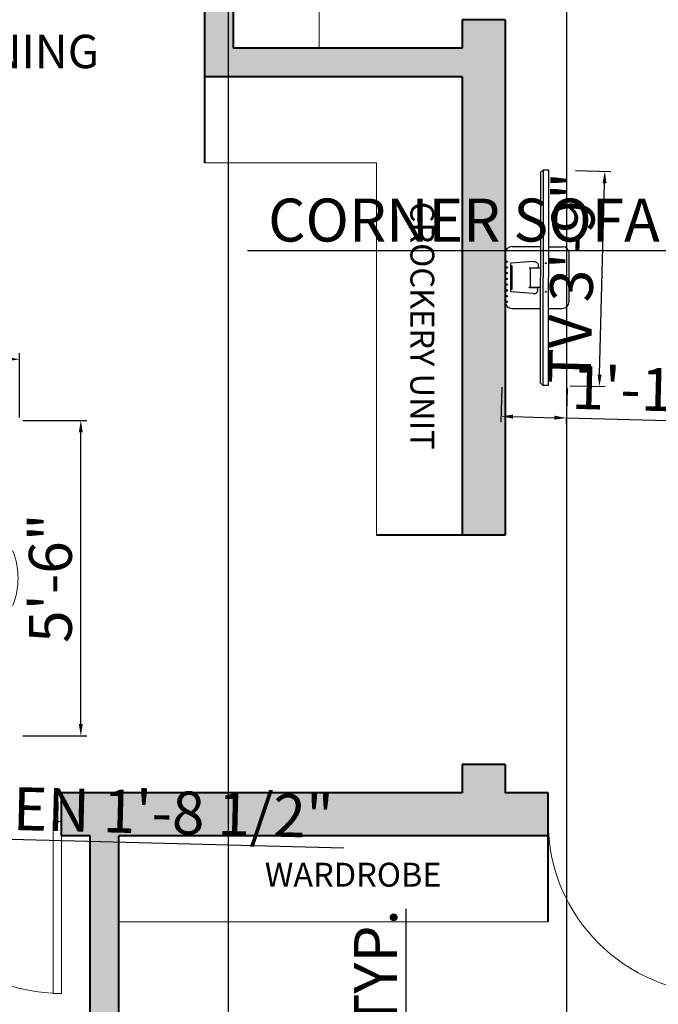
# Model space of a CAD drawing. Units: inches. Extents: x 2337 to 3570, y 1258 to 1938.
# Tile 4 of 30: x 2570 to 2704, y 1507 to 1713. Entities that reach past the tile are written whole.
import ezdxf

# ---------------------------------------------------------------- set-up
doc = ezdxf.new("R2010")
doc.units = ezdxf.units.IN
for name, color, linetype, lineweight in [('A-ANNO-DIMS', 2, 'Continuous', 18), ('A-ANNO-TEXT', 7, 'Continuous', 18), ('A-AREA-IDEN', 7, 'Continuous', 18), ('A-DOOR', 4, 'Continuous', 20), ('A-EQPM', 9, 'Continuous', 18), ('A-FLOR-CASE', 34, 'Continuous', 18), ('A-WALL', 7, 'Continuous', 40), ('furn', 8, 'Continuous', 18)]:
    doc.layers.add(name, color=color, linetype=linetype, lineweight=lineweight)
doc.layers.add('A-WALL-PATT', color=18, linetype='Continuous', lineweight=13, true_color=0x000000)
doc.layers.add('window', color=130, linetype='Continuous')
doc.styles.get("Standard").update_dxf_attribs({"font": 'arial.ttf'})
doc.dimstyles.new('ISO-25', dxfattribs={"dimtxt": 9, "dimasz": 2.5, "dimexe": 1.25, "dimexo": 0.625, "dimtad": 1, "dimdec": 1, "dimlunit": 3, "dimtxsty": 'Standard', "dimcen": 2.5, "dimadec": 0, "dimazin": 0, "dimtfac": 1, "dimtdec": 1, "dimtmove": 0, "dimatfit": 3, "dimfxl": 1, "dimarcsym": 0})

# ---------------------------------------------------------------- blocks, each defined once
blk = doc.blocks.new('*U2')
for p, q in [((0, 0), (0, -6)), ((36, 0), (36, -6))]:
    blk.add_line(p, q)
blk.add_lwpolyline([(0, 0), (0, 36), (1.75, 36), (1.75, 0)], close=True)
blk.add_arc((0, 0), 36, 0, 90)
blk = doc.blocks.new('table-23')
at = {"color": 0, "linetype": 'ByBlock'}
for p, q in [((-0.6323, 0.4685), (-0.6236, 0.5245)), ((-0.2677, 0.4685), (-0.2764, 0.5245)), ((-0.485, 0.5057), (-0.485, 0.4355)), ((-0.415, 0.5057), (-0.415, 0.4355)), ((-0.675, 0.107), (-0.645, 0.387)), ((-0.225, 0.107), (-0.255, 0.387)), ((-0.9, -1.4923), (-0.9, 0)), ((-0.9, 0), (0, 0)), ((0, -1.4923), (0, 0)), ((-1.0062, -0.2211), (-1.2862, -0.2511)), ((0.1062, -0.2211), (0.3862, -0.2511)), ((-1.3677, -0.2639), (-1.4237, -0.2726)), ((0.4677, -0.2639), (0.5237, -0.2726)), ((-1.4049, -0.4111), (-1.3347, -0.4111)), ((0.5049, -0.4111), (0.4347, -0.4111)), ((-1.4049, -0.4811), (-1.3347, -0.4811)), ((0.5049, -0.4811), (0.4347, -0.4811)), ((-1.3677, -0.6284), (-1.4237, -0.6197)), ((0.4677, -0.6284), (0.5237, -0.6197)), ((-1.0062, -0.6711), (-1.2862, -0.6411)), ((0.1062, -0.6711), (0.3862, -0.6411)), ((-1.0062, -0.8211), (-1.2862, -0.8511)), ((0.1062, -0.8211), (0.3862, -0.8511)), ((-1.3677, -0.8639), (-1.4237, -0.8726)), ((0.4677, -0.8639), (0.5237, -0.8726)), ((-1.4049, -1.0111), (-1.3347, -1.0111)), ((0.5049, -1.0111), (0.4347, -1.0111)), ((-1.4049, -1.0811), (-1.3347, -1.0811)), ((0.5049, -1.0811), (0.4347, -1.0811)), ((-1.3677, -1.2284), (-1.4237, -1.2197)), ((-1.0062, -1.2711), (-1.2862, -1.2411)), ((0.1062, -1.2711), (0.3862, -1.2411)), ((0.4677, -1.2284), (0.5237, -1.2197)), ((-0.9, -1.4923), (0, -1.4923)), ((-0.675, -1.5993), (-0.645, -1.8793)), ((-0.225, -1.5993), (-0.255, -1.8793)), ((-0.6323, -1.9608), (-0.6236, -2.0168)), ((-0.485, -1.998), (-0.485, -1.9278)), ((-0.415, -1.998), (-0.415, -1.9278)), ((-0.2677, -1.9608), (-0.2764, -2.0168))]:
    blk.add_line(p, q, dxfattribs=at)
for centre, radius, start, end in [((-0.45, 0.0773), 0.4797, 68.78869, 111.21131), ((-0.45, 0.0566), 0.4505, 66.13443, 113.86557), ((-0.45, 0.0318), 0.4053, 61.23721, 118.76279), ((-0.45, 0.5883), 0.5312, 244.94238, 295.05762), ((-0.931, -0.4461), 0.4053, 151.23721, 208.76279), ((-1.4875, -0.4461), 0.5312, 334.94238, 25.05762), ((0.5875, -0.4461), 0.5312, 154.94238, 205.05762), ((0.031, -0.4461), 0.4053, 331.23721, 28.76279), ((-0.9765, -0.4461), 0.4797, 158.78869, 201.21131), ((-0.9558, -0.4461), 0.4505, 156.13443, 203.86557), ((0.0558, -0.4461), 0.4505, 336.13443, 23.86557), ((0.0765, -0.4461), 0.4797, 338.78869, 21.21131), ((-1.4875, -1.0461), 0.5312, 334.94238, 25.05762), ((0.5875, -1.0461), 0.5312, 154.94238, 205.05762), ((-0.9765, -1.0461), 0.4797, 158.78869, 201.21131), ((-0.9558, -1.0461), 0.4505, 156.13443, 203.86557), ((-0.931, -1.0461), 0.4053, 151.23721, 208.76279), ((0.031, -1.0461), 0.4053, 331.23721, 28.76279), ((0.0558, -1.0461), 0.4505, 336.13443, 23.86557), ((0.0765, -1.0461), 0.4797, 338.78869, 21.21131), ((-0.45, -2.0806), 0.5312, 64.94238, 115.05762), ((-0.45, -1.5241), 0.4053, 241.23721, 298.76279), ((-0.45, -1.5489), 0.4505, 246.13443, 293.86557), ((-0.45, -1.5696), 0.4797, 248.78869, 291.21131)]:
    blk.add_arc(centre, radius, start, end, dxfattribs=at)
blk = doc.blocks.new('TV')
at = {"color": 0}
for p, q in [((3967.269, 1784.848), (3967.048, 1784.654)), ((3967.765, 1763.677), (3967.535, 1763.861))]:
    blk.add_line(p, q, dxfattribs=at)
at = {"layer": 'window'}
for p, q in [((3967.535, 1763.861), (3967.048, 1784.654)), ((3964.405, 1777.232), (3967.221, 1777.298)), ((3968.009, 1777.316), (3969.36, 1777.348)), ((3966.535, 1775.819), (3964.331, 1775.605)), ((3964.337, 1775.337), (3964.45, 1775.34)), ((3964.337, 1775.315), (3964.428, 1775.317)), ((3966.143, 1775.199), (3967.01, 1775.22)), ((3966.144, 1775.177), (3966.143, 1775.199)), ((3966.144, 1775.177), (3967.27, 1775.203)), ((3966.3, 1773.288), (3966.256, 1775.179)), ((3964.39, 1773.063), (3964.48, 1773.065)), ((3966.188, 1773.285), (3967.314, 1773.311)), ((3966.188, 1773.262), (3966.188, 1773.285)), ((3966.188, 1773.262), (3967.055, 1773.283)), ((3964.391, 1773.04), (3964.503, 1773.043)), ((3966.608, 1772.662), (3964.397, 1772.772)), ((3964.548, 1771.151), (3967.363, 1771.217)), ((3968.151, 1771.235), (3969.503, 1771.267))]:
    blk.add_line(p, q, dxfattribs=at)
for points in [[(3968.328, 1763.69), (3967.832, 1784.861), (3967.269, 1784.848), (3967.765, 1763.677), (3968.328, 1763.69)], [(3963.856, 1771.811), (3963.745, 1776.54)], [(3970.163, 1771.958), (3970.052, 1776.688)], [(3964.397, 1772.772), (3964.331, 1775.605)], [(3964.48, 1773.065), (3964.428, 1775.317)], [(3964.503, 1773.043), (3964.45, 1775.34)]]:
    blk.add_lwpolyline(points, dxfattribs=at)
for points in [[(3966.535, 1775.819, -0.263666), (3966.933, 1775.689), (3967.001, 1775.572), (3967.01, 1775.22)], [(3966.608, 1772.662, 0.263666), (3967, 1772.811), (3967.063, 1772.93), (3967.055, 1773.283)]]:
    blk.add_lwpolyline(points, format="xyb", dxfattribs=at)
for centre, radius in [((3963.914, 1775.731), 0.0679), ((3963.927, 1775.168), 0.0679), ((3967.766, 1775.678), 0.0451), ((3963.94, 1774.605), 0.0679), ((3963.953, 1774.042), 0.0679), ((3963.966, 1773.478), 0.0679), ((3963.979, 1772.915), 0.0679), ((3963.993, 1772.352), 0.0679), ((3967.832, 1772.86), 0.0451), ((3964.006, 1771.789), 0.0679)]:
    blk.add_circle(centre, radius, dxfattribs=at)
for centre, start, end in [((3964.421, 1776.556), 91.34137, 181.34137), ((3969.376, 1776.672), 1.34137, 91.34137), ((3964.532, 1771.826), 181.34137, 271.34137), ((3969.487, 1771.942), 271.34137, 1.34137)]:
    blk.add_arc(centre, 0.676, start, end, dxfattribs=at)
blk = doc.blocks.new('*D54')
at = {"layer": 'A-ANNO-DIMS', "color": 0, "lineweight": -2, "transparency": 16777216}
for p, q in [((2686.58, 1681.49), (2693.96, 1681.3)), ((2691.63, 1638.77), (2692.65, 1678.83)), ((2685.43, 1636.42), (2692.82, 1636.24))]:
    blk.add_line(p, q, dxfattribs=at)
at = {"layer": 'A-ANNO-DIMS', "color": 0, "transparency": 16777216}
for points in [[(2692.23, 1678.84), (2693.07, 1678.82), (2692.71, 1681.33)], [(2691.21, 1638.78), (2692.05, 1638.76), (2691.57, 1636.27)]]:
    blk.add_solid(points, dxfattribs=at)
at = {"layer": 'Defpoints', "color": 0, "transparency": 16777216}
for p in [(2685.95, 1681.5), (2692.71, 1681.33), (2684.81, 1636.44)]:
    blk.add_point(p, dxfattribs=at)
at = {"layer": 'A-ANNO-DIMS', "color": 0, "transparency": 16777216, "insert": (2686.92, 1658.93), "char_height": 9, "attachment_point": 5, "rotation": 88.5431}
blk.add_mtext('TV 3\'-9"', dxfattribs=at)
blk = doc.blocks.new('*D55')
at = {"layer": 'A-ANNO-DIMS', "color": 0, "lineweight": -2, "transparency": 16777216}
for p, q in [((2671.13, 1636.16), (2670.94, 1628.78)), ((2684.79, 1635.82), (2684.6, 1628.43)), ((2673.47, 1629.97), (2682.14, 1629.74)), ((2684.64, 1629.68), (2732.42, 1628.47))]:
    blk.add_line(p, q, dxfattribs=at)
at = {"layer": 'A-ANNO-DIMS', "color": 0, "transparency": 16777216}
for points in [[(2673.48, 1630.38), (2673.46, 1629.55), (2670.97, 1630.03)], [(2682.15, 1630.16), (2682.13, 1629.33), (2684.64, 1629.68)]]:
    blk.add_solid(points, dxfattribs=at)
at = {"layer": 'Defpoints', "color": 0, "transparency": 16777216}
for p in [(2671.14, 1636.79), (2684.81, 1636.44), (2684.64, 1629.68)]:
    blk.add_point(p, dxfattribs=at)
at = {"layer": 'A-ANNO-DIMS', "color": 0, "transparency": 16777216, "insert": (2709.91, 1634.32), "char_height": 9, "attachment_point": 5, "rotation": 358.5431}
blk.add_mtext('1\'-1 1/2"', dxfattribs=at)
blk = doc.blocks.new('*D56')
at = {"layer": 'A-ANNO-DIMS', "color": 0, "lineweight": -2, "transparency": 16777216}
for p, q in [((2512.75, 1540.36), (2512.84, 1544.09)), ((2533.46, 1539.83), (2533.56, 1543.56)), ((2515.31, 1542.78), (2531.03, 1542.38)), ((2533.53, 1542.31), (2637.99, 1539.66))]:
    blk.add_line(p, q, dxfattribs=at)
at = {"layer": 'A-ANNO-DIMS', "color": 0, "transparency": 16777216}
for points in [[(2515.32, 1543.19), (2515.3, 1542.36), (2512.81, 1542.84)], [(2531.04, 1542.79), (2531.02, 1541.96), (2533.53, 1542.31)]]:
    blk.add_solid(points, dxfattribs=at)
at = {"layer": 'Defpoints', "color": 0, "transparency": 16777216}
for p in [(2533.53, 1542.31), (2512.73, 1539.73), (2533.45, 1539.2)]:
    blk.add_point(p, dxfattribs=at)
at = {"layer": 'A-ANNO-DIMS', "color": 0, "transparency": 16777216, "insert": (2587.14, 1546.23), "char_height": 9, "attachment_point": 5, "rotation": 358.5431}
blk.add_mtext('SCREEN 1\'-8 1/2"', dxfattribs=at)
blk = doc.blocks.new('*D67')
at = {"layer": 'A-ANNO-DIMS', "color": 0, "lineweight": -2, "transparency": 16777216}
for p, q in [((2651.1, 1448.1), (2651.1, 1526.84)), ((2653.98, 1448.1), (2649.85, 1448.1)), ((2651.1, 1435.25), (2651.1, 1445.6)), ((2653.98, 1432.75), (2649.85, 1432.75))]:
    blk.add_line(p, q, dxfattribs=at)
at = {"layer": 'A-ANNO-DIMS', "color": 0, "transparency": 16777216}
for points in [[(2650.68, 1445.6), (2651.52, 1445.6), (2651.1, 1448.1)], [(2650.68, 1435.25), (2651.52, 1435.25), (2651.1, 1432.75)]]:
    blk.add_solid(points, dxfattribs=at)
at = {"layer": 'Defpoints', "color": 0, "transparency": 16777216}
for p in [(2651.1, 1448.1), (2654.61, 1448.1), (2654.61, 1432.75)]:
    blk.add_point(p, dxfattribs=at)
at = {"layer": 'A-ANNO-DIMS', "color": 0, "transparency": 16777216, "insert": (2645.82, 1488.72), "char_height": 9, "attachment_point": 5, "rotation": 90}
blk.add_mtext('1\'-3 1/2" TYP.', dxfattribs=at)
blk = doc.blocks.new('*D78')
at = {"layer": 'A-ANNO-DIMS', "color": 0, "lineweight": -2, "transparency": 16777216}
for p, q in [((2484.66, 1641.99), (2361.02, 1641.99)), ((2484.66, 1629.8), (2484.66, 1643.24)), ((2567.57, 1641.99), (2487.16, 1641.99)), ((2570.07, 1629.8), (2570.07, 1643.24))]:
    blk.add_line(p, q, dxfattribs=at)
at = {"layer": 'A-ANNO-DIMS', "color": 0, "transparency": 16777216}
for points in [[(2487.16, 1642.4), (2487.16, 1641.57), (2484.66, 1641.99)], [(2567.57, 1642.4), (2567.57, 1641.57), (2570.07, 1641.99)]]:
    blk.add_solid(points, dxfattribs=at)
at = {"layer": 'Defpoints', "color": 0, "transparency": 16777216}
for p in [(2484.66, 1641.99), (2484.66, 1629.18), (2570.07, 1629.18)]:
    blk.add_point(p, dxfattribs=at)
at = {"layer": 'A-ANNO-DIMS', "color": 0, "transparency": 16777216, "insert": (2421.59, 1647.27), "char_height": 9, "attachment_point": 5}
blk.add_mtext('DINING SET 7\'-1 1/2"', dxfattribs=at)
blk = doc.blocks.new('*D79')
at = {"layer": 'A-ANNO-DIMS', "color": 0, "lineweight": -2, "transparency": 16777216}
for p, q in [((2570.7, 1629.18), (2584.14, 1629.18)), ((2582.89, 1565.57), (2582.89, 1626.68)), ((2570.7, 1563.07), (2584.14, 1563.07))]:
    blk.add_line(p, q, dxfattribs=at)
at = {"layer": 'A-ANNO-DIMS', "color": 0, "transparency": 16777216}
for points in [[(2582.47, 1626.68), (2583.3, 1626.68), (2582.89, 1629.18)], [(2582.47, 1565.57), (2583.3, 1565.57), (2582.89, 1563.07)]]:
    blk.add_solid(points, dxfattribs=at)
at = {"layer": 'Defpoints', "color": 0, "transparency": 16777216}
for p in [(2570.07, 1629.18), (2582.89, 1629.18), (2570.07, 1563.07)]:
    blk.add_point(p, dxfattribs=at)
at = {"layer": 'A-ANNO-DIMS', "color": 0, "transparency": 16777216, "insert": (2577.67, 1596.12), "char_height": 9, "attachment_point": 5, "rotation": 90}
blk.add_mtext('5\'-6"', dxfattribs=at)
blk = doc.blocks.new('*D86')
at = {"layer": 'A-ANNO-DIMS', "color": 0, "lineweight": -2, "transparency": 16777216}
for p, q in [((2762.09, 1679.33), (2762.09, 1663.44)), ((2863.84, 1679.33), (2863.84, 1663.44)), ((2762.09, 1664.69), (2617.85, 1664.69)), ((2861.34, 1664.69), (2764.59, 1664.69))]:
    blk.add_line(p, q, dxfattribs=at)
at = {"layer": 'A-ANNO-DIMS', "color": 0, "transparency": 16777216}
for points in [[(2764.59, 1665.11), (2764.59, 1664.28), (2762.09, 1664.69)], [(2861.34, 1665.11), (2861.34, 1664.28), (2863.84, 1664.69)]]:
    blk.add_solid(points, dxfattribs=at)
at = {"layer": 'Defpoints', "color": 0, "transparency": 16777216}
for p in [(2762.09, 1679.95), (2863.84, 1679.95), (2762.09, 1664.69)]:
    blk.add_point(p, dxfattribs=at)
at = {"layer": 'A-ANNO-DIMS', "color": 0, "transparency": 16777216, "insert": (2688.72, 1669.97), "char_height": 9, "attachment_point": 5}
blk.add_mtext('CORNER SOFA 8\'-5 1/2"', dxfattribs=at)
blk = doc.blocks.new('*D118')
at = {"layer": 'A-ANNO-DIMS', "color": 0, "lineweight": -2, "transparency": 16777216}
for p, q in [((2613.87, 1497.86), (2613.87, 1927.77)), ((2684.73, 1497.86), (2684.73, 1927.77)), ((2616.37, 1926.52), (2682.23, 1926.52))]:
    blk.add_line(p, q, dxfattribs=at)
at = {"layer": 'A-ANNO-DIMS', "color": 0, "transparency": 16777216}
for points in [[(2616.37, 1926.93), (2616.37, 1926.1), (2613.87, 1926.52)], [(2682.23, 1926.93), (2682.23, 1926.1), (2684.73, 1926.52)]]:
    blk.add_solid(points, dxfattribs=at)
at = {"layer": 'Defpoints', "color": 0, "transparency": 16777216}
for p in [(2684.73, 1926.52), (2613.87, 1497.23), (2684.73, 1497.23)]:
    blk.add_point(p, dxfattribs=at)
at = {"layer": 'A-ANNO-DIMS', "color": 0, "transparency": 16777216, "insert": (2649.3, 1931.74), "char_height": 9, "attachment_point": 5}
blk.add_mtext('5\'-11"', dxfattribs=at)

msp = doc.modelspace()

# ---------------------------------------------------------------- hatches: boundary and pattern name
at = {"layer": 'A-WALL-PATT'}
h = msp.add_hatch(color=256, dxfattribs=at)
h.dxf.hatch_style = 1
h.paths.add_polyline_path([(2671.84, 1857.12), (2455.84, 1857.12), (2455.84, 1824.12), (2464.84, 1824.12), (2464.84, 1848.12), (2671.84, 1848.12)])
h.paths.add_polyline_path([(2566.84, 1764.12), (2464.84, 1764.12), (2464.84, 1788.12), (2455.84, 1788.12), (2455.84, 1743.12), (2464.84, 1743.12), (2464.84, 1755.12), (2566.84, 1755.12)])
h.paths.add_polyline_path([(2683.84, 1761.12), (2683.84, 1764.12), (2602.84, 1764.12), (2602.84, 1755.12), (2608.84, 1755.12), (2608.84, 1701.12), (2662.84, 1701.12), (2662.84, 1605.12), (2671.84, 1605.12), (2671.84, 1713.12), (2662.84, 1713.12), (2662.84, 1707.12), (2614.84, 1707.12), (2614.84, 1755.12), (2662.84, 1755.12), (2662.84, 1749.12), (2671.84, 1749.12), (2671.84, 1755.12), (2683.84, 1755.12)])
h.paths.add_polyline_path([(2464.84, 1707.12), (2455.84, 1707.12), (2455.84, 1617.12), (2464.84, 1617.12), (2464.84, 1635.12), (2506.84, 1635.12), (2506.84, 1641.12), (2464.84, 1641.12)])
h.paths.add_polyline_path([(2542.84, 1551.12), (2464.84, 1551.12), (2464.84, 1569.12), (2455.84, 1569.12), (2455.84, 1518.12), (2464.84, 1518.12), (2464.84, 1542.12), (2542.84, 1542.12)])
h.paths.add_polyline_path([(2464.84, 1482.12), (2455.84, 1482.12), (2455.84, 1410.12), (2464.84, 1410.12)])
h.paths.add_polyline_path([(2626.84, 1350.12), (2590.84, 1350.12), (2590.84, 1380.12), (2584.84, 1380.12), (2584.84, 1350.12), (2464.84, 1350.12), (2464.84, 1374.12), (2455.84, 1374.12), (2455.84, 1341.12), (2626.84, 1341.12)])
h.paths.add_polyline_path([(2662.84, 1416.12), (2686.84, 1416.12), (2686.84, 1422.12), (2590.84, 1422.12), (2590.84, 1542.12), (2680.84, 1542.12), (2680.84, 1551.12), (2671.84, 1551.12), (2671.84, 1557.12), (2662.84, 1557.12), (2662.84, 1551.12), (2578.84, 1551.12), (2578.84, 1542.12), (2584.84, 1542.12), (2584.84, 1410.12), (2590.84, 1410.12), (2590.84, 1416.12), (2656.84, 1416.12), (2656.84, 1350.12), (2650.84, 1350.12), (2650.84, 1341.12), (2731.84, 1341.12), (2731.84, 1362.12), (2722.84, 1362.12), (2722.84, 1350.12), (2662.84, 1350.12)])
h.paths.add_polyline_path([(2731.84, 1434.12), (2722.84, 1434.12), (2722.84, 1422.12), (2716.84, 1422.12), (2716.84, 1416.12), (2722.84, 1416.12), (2722.84, 1386.12), (2731.84, 1386.12)], flags=17)
h.paths.add_polyline_path([(2731.84, 1542.12), (2752.84, 1542.12), (2752.84, 1551.12), (2716.84, 1551.12), (2716.84, 1545.12), (2716.84, 1542.12), (2722.84, 1542.12), (2722.84, 1482.12), (2731.84, 1482.12)])
h.paths.add_polyline_path([(2809.84, 1551.12), (2788.84, 1551.12), (2788.84, 1542.12), (2809.84, 1542.12), (2809.84, 1548.12)])
h.paths.add_polyline_path([(2872.84, 1647.12), (2863.84, 1647.12), (2863.84, 1551.12), (2857.84, 1551.12), (2857.84, 1548.12), (2857.84, 1542.12), (2872.84, 1542.12)])
h.paths.add_polyline_path([(2872.84, 1764.12), (2827.84, 1764.12), (2827.84, 1755.12), (2863.84, 1755.12), (2863.84, 1719.12), (2872.84, 1719.12)])
h.paths.add_polyline_path([(2755.84, 1764.12), (2719.84, 1764.12), (2719.84, 1755.12), (2755.84, 1755.12)])

# ---------------------------------------------------------------- linework, layer by layer
at = {"layer": 'A-FLOR-CASE'}
for p, q in [((2632.84, 1755.12), (2632.84, 1707.12)), ((2644.84, 1683.12), (2608.84, 1683.12)), ((2644.84, 1683.12), (2644.84, 1605.12)), ((2680.84, 1524.12), (2590.84, 1524.12))]:
    msp.add_line(p, q, dxfattribs=at)
at = {"layer": 'A-WALL'}
for p, q in [((2608.84, 1755.12), (2608.84, 1683.12)), ((2614.84, 1755.12), (2614.84, 1707.12)), ((2662.84, 1713.12), (2662.84, 1707.12)), ((2671.84, 1713.12), (2662.84, 1713.12)), ((2671.84, 1713.12), (2671.84, 1605.12)), ((2662.84, 1707.12), (2614.84, 1707.12)), ((2662.84, 1701.12), (2608.84, 1701.12)), ((2662.84, 1701.12), (2662.84, 1605.12)), ((2671.84, 1605.12), (2644.84, 1605.12)), ((2662.84, 1557.12), (2662.84, 1551.12)), ((2671.84, 1557.12), (2662.84, 1557.12)), ((2671.84, 1557.12), (2671.84, 1551.12)), ((2662.84, 1551.12), (2578.84, 1551.12)), ((2578.84, 1542.12), (2578.84, 1551.12)), ((2680.84, 1551.12), (2671.84, 1551.12)), ((2680.84, 1524.12), (2680.84, 1551.12)), ((2584.84, 1542.12), (2578.84, 1542.12)), ((2584.84, 1410.12), (2584.84, 1542.12)), ((2680.84, 1542.12), (2590.84, 1542.12)), ((2590.84, 1422.12), (2590.84, 1542.12))]:
    msp.add_line(p, q, dxfattribs=at)

# ---------------------------------------------------------------- block references
at = {"layer": 'A-DOOR', "rotation": 180}
for p in [(2578.84, 1545.12), (2716.84, 1545.12)]:
    msp.add_blockref('*U2', p, dxfattribs=at)
at = {"layer": 'A-EQPM', "xscale": 2.127748957344282, "yscale": 2.127748957344282, "zscale": 2.127748957344282, "rotation": 358.5430845181614}
msp.add_blockref('TV', (-5855.39, -1900.23), dxfattribs=at)
at = {"layer": 'furn', "xscale": 32.50065408352129, "yscale": 32.50065408352129, "zscale": 32.50065408352129, "rotation": 90}
msp.add_blockref('table-23', (2503.12, 1610.75), dxfattribs=at)

# ---------------------------------------------------------------- texts
at = {"layer": 'A-ANNO-TEXT', "insert": (2656.97, 1674.98), "char_height": 5, "attachment_point": 1, "rotation": 270}
msp.add_mtext_dynamic_manual_height_columns('CROCKERY UNIT', width=66.911, gutter_width=12.5, heights=[0], dxfattribs=at)
at = {"layer": 'A-ANNO-TEXT', "insert": (2621.44, 1536.5), "char_height": 5, "attachment_point": 1}
msp.add_mtext_dynamic_manual_height_columns('WARDROBE', width=66.911, gutter_width=12.5, heights=[0], dxfattribs=at)
at = {"layer": 'A-AREA-IDEN', "insert": (2508.61, 1709.96), "char_height": 7, "attachment_point": 1}
msp.add_mtext_dynamic_manual_height_columns('KITCHEN+DINING\\P     11\'6"X9\'6"', width=66.911, gutter_width=12.5, heights=[0], dxfattribs=at)

# ---------------------------------------------------------------- dimensions: what is measured, and where the dimension line sits
at = {"layer": 'A-ANNO-DIMS'}
dim = msp.add_linear_dim(base=(2684.73, 1926.52), p1=(2613.87, 1497.23), p2=(2684.73, 1497.23), dimstyle='ISO-25', override={"dimdec": 1, "dimlfac": 1, "dimrnd": 0, "dimzin": 1, "dimdsep": 46, "dimlunit": 4, "dimfrac": 2}, dxfattribs=at)
dim.commit()
dim.dimension.update_dxf_attribs({"geometry": '*D118', "text_midpoint": (2649.3, 1931.74)})
for base, p1, p2, angle, text, picture, middle in [((2762.0922, 1664.6925), (2863.8358, 1679.9541), (2762.0922, 1679.9541), 180, 'CORNER SOFA <>', '*D86', (2688.7199, 1669.9741)), ((2692.71, 1681.33), (2684.81, 1636.44), (2685.95, 1681.5), 88.5431, 'TV <>', '*D54', (2686.92, 1658.93)), ((2484.66, 1641.99), (2570.07, 1629.18), (2484.66, 1629.18), 180, 'DINING SET <>', '*D78', (2421.59, 1647.27)), ((2533.53, 1542.31), (2512.73, 1539.73), (2533.45, 1539.2), 358.5431, 'SCREEN <>', '*D56', (2587.14, 1546.23)), ((2651.1014, 1448.1023), (2654.6093, 1432.748), (2654.6093, 1448.1023), 90, '<> TYP.', '*D67', (2645.8199, 1488.7191))]:
    dim = msp.add_linear_dim(base=base, p1=p1, p2=p2, angle=angle, text=text, dimstyle='ISO-25', override={"dimdec": 1, "dimlfac": 1, "dimrnd": 0, "dimzin": 1, "dimdsep": 46, "dimlunit": 4, "dimfrac": 2}, dxfattribs=at)
    dim.commit()
    dim.dimension.update_dxf_attribs({"geometry": picture, "text_midpoint": middle})
for base, p1, p2, angle, picture, middle in [((2684.64, 1629.68), (2671.14, 1636.79), (2684.81, 1636.44), 358.5431, '*D55', (2709.91, 1634.32)), ((2582.89, 1629.18), (2570.07, 1563.07), (2570.07, 1629.18), 90, '*D79', (2577.67, 1596.12))]:
    dim = msp.add_linear_dim(base=base, p1=p1, p2=p2, angle=angle, dimstyle='ISO-25', override={"dimdec": 1, "dimlfac": 1, "dimrnd": 0, "dimzin": 1, "dimdsep": 46, "dimlunit": 4, "dimfrac": 2}, dxfattribs=at)
    dim.commit()
    dim.dimension.update_dxf_attribs({"geometry": picture, "text_midpoint": middle})

doc.saveas('drawing.dxf')
